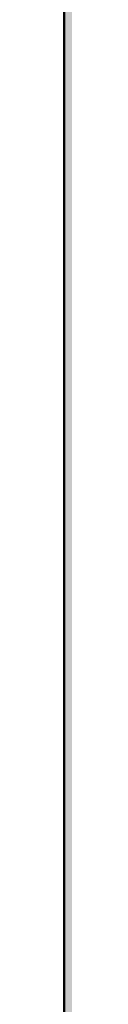
# Model space of a CAD drawing. Units: millimetres. Extents: x 0 to 2267, y 0 to 1823.
# Tile 33 of 256: x 1593.4289 to 1593.4289, y 1226.3857 to 1226.718. Entities that reach past the tile are written whole.
import ezdxf

# ---------------------------------------------------------------- set-up
doc = ezdxf.new("R2010")
doc.units = ezdxf.units.MM
doc.header["$MEASUREMENT"] = 0
doc.layers.add('M-HATC', color=252, linetype='Continuous', lineweight=18)
doc.layers.add('M-OUTL', color=7, linetype='Continuous', lineweight=50)

msp = doc.modelspace()

# ---------------------------------------------------------------- hatches: boundary and pattern name
at = {"layer": 'M-HATC'}
h = msp.add_hatch(color=256, dxfattribs=at)
h.dxf.hatch_style = 1
h.paths.add_polyline_path([(2055.77105, 1603.06204), (1381.08677, 1603.06204), (1381.08677, 1598.06204), (2055.77105, 1598.06204)])
h.paths.add_polyline_path([(2055.77105, 1598.06204), (1381.08677, 1598.06204), (1381.08677, 1593.06204), (2055.77105, 1593.06204)])
h.paths.add_polyline_path([(2051.30737, 1536.76088), (1385.55044, 1536.76088), (1385.55044, 1526.76088), (1387.55044, 1526.76088), (1388.53662, 1525.05276), (1385.33187, 1521.23348), (1385.33187, 1521.22256), (2050.25417, 1522.74913), (2048.32119, 1525.05276), (2049.30737, 1526.76088), (2051.30737, 1526.76088)])
edge = h.paths.add_edge_path()
edge.add_arc((1847.53451, 1379.14917), 135, 222.6030607, 222.8908505, ccw=False)
edge.add_line((1748.16629, 1287.76561), (1683.09212, 1287.76561))
edge.add_arc((1583.7239, 1379.14917), 135, 317.1091495, 317.3969393, ccw=False)
edge.add_arc((1678.9686, 1290.67067), 5, 222.89085, 317.10915, ccw=False)
edge.add_arc((1774.21331, 1379.14917), 135, 222.6030607, 222.8908505, ccw=False)
edge.add_line((1674.84509, 1287.76561), (1609.77092, 1287.76561))
edge.add_arc((1510.4027, 1379.14917), 135, 317.1091495, 317.3969393, ccw=False)
edge.add_arc((1605.6474, 1290.67067), 5, 222.89085, 317.10915, ccw=False)
edge.add_arc((1700.89211, 1379.14917), 135, 222.6030607, 222.8908505, ccw=False)
edge.add_line((1601.52388, 1287.76561), (1536.44972, 1287.76561))
edge.add_arc((1437.08149, 1379.14917), 135, 317.1091495, 317.3969393, ccw=False)
edge.add_arc((1532.3262, 1290.67067), 5, 222.89085, 317.10915, ccw=False)
edge.add_arc((1627.57091, 1379.14917), 135, 222.6030607, 222.8908505, ccw=False)
edge.add_line((1528.20268, 1287.76561), (1505.92891, 1287.76561))
edge.add_spline(control_points=[(1505.92891, 1287.76561), (1504.26224, 1287.76561), (1504.26224, 1282.76561), (1505.92891, 1282.76561)], knot_values=[0, 0, 0, 0, 5, 5, 5, 5], degree=3, periodic=0)
edge.add_line((1505.92891, 1282.76561), (1930.92891, 1282.76561))
edge.add_spline(control_points=[(1930.92891, 1282.76561), (1932.59557, 1282.76561), (1932.59557, 1287.76561), (1930.92891, 1287.76561)], knot_values=[0, 0, 0, 0, 5, 5, 5, 5], degree=3, periodic=0)
edge.add_line((1930.92891, 1287.76561), (1903.05573, 1287.76561))
edge.add_arc((1803.6875, 1379.14917), 135, 317.1091495, 317.3969393, ccw=False)
edge.add_arc((1898.93221, 1290.67067), 5, 222.89085, 317.10915, ccw=False)
edge.add_arc((1994.17691, 1379.14917), 135, 222.6030607, 222.8908505, ccw=False)
edge.add_line((1894.80869, 1287.76561), (1829.73452, 1287.76561))
edge.add_arc((1730.3663, 1379.14917), 135, 317.1091495, 317.3969393, ccw=False)
edge.add_arc((1825.61101, 1290.67067), 5, 222.89085, 317.10915, ccw=False)
edge.add_arc((1920.85571, 1379.14917), 135, 222.6030607, 222.8908505, ccw=False)
edge.add_line((1821.48749, 1287.76561), (1756.41332, 1287.76561))
edge.add_arc((1657.0451, 1379.14917), 135, 317.1091495, 317.3969393, ccw=False)
edge.add_arc((1752.28981, 1290.67067), 5, 222.89085, 317.10915, ccw=False)
edge = h.paths.add_edge_path()
edge.add_spline(control_points=[(1843.42891, 1227.24746), (1845.09557, 1227.24746), (1845.09557, 1232.24746), (1843.42891, 1232.24746)], knot_values=[0, 0, 0, 0, 5, 5, 5, 5], degree=3, periodic=0)
edge.add_line((1843.42891, 1232.24746), (1593.42891, 1232.24746))
edge.add_spline(control_points=[(1593.42891, 1232.24746), (1591.76224, 1232.24746), (1591.76224, 1227.24746), (1593.42891, 1227.24746)], knot_values=[0, 0, 0, 0, 5, 5, 5, 5], degree=3, periodic=0)
edge.add_line((1593.42891, 1227.24746), (1843.42891, 1227.24746))
h.paths.add_polyline_path([(1905.92891, 1127.41706), (1530.92891, 1127.41706, 0.414214), (1520.92891, 1117.41706), (1530.92891, 1117.41706), (1915.92891, 1117.41706, 0.414214)])
edge = h.paths.add_edge_path()
edge.add_arc((1397.08577, 1498.40775), 12.72993, 90.782146, 190.878706, ccw=False)
edge.add_line((1396.912, 1511.13649), (1428.00968, 1511.34875))
edge.add_line((1428.00968, 1511.34875), (1433.00968, 1511.34875))
edge.add_line((1433.00968, 1511.34875), (1434.439, 1511.34875))
edge.add_arc((1419.474, 1498.08041), 20, 41.560995, 74.082109)
edge.add_line((1424.95919, 1517.31353), (1399.93509, 1517.25608))
edge.add_spline(control_points=[(1399.93074, 1517.25607), (1399.88398, 1517.21312), (1399.8328, 1517.16893), (1399.77741, 1517.1236)], knot_values=[11.567499, 11.567499, 11.567499, 11.567499, 11.814249, 11.814249, 11.814249, 11.814249], degree=3, periodic=0)
edge.add_spline(control_points=[(1399.63279, 1517.00986), (1399.58305, 1516.97214), (1399.53072, 1516.93375), (1399.47591, 1516.89474)], knot_values=[11.167718, 11.167718, 11.167718, 11.167718, 11.365188, 11.365188, 11.365188, 11.365188], degree=3, periodic=0)
edge.add_spline(control_points=[(1399.33981, 1516.80007), (1399.15144, 1516.67185), (1398.93836, 1516.5377), (1398.70404, 1516.39942)], knot_values=[10.376405, 10.376405, 10.376405, 10.376405, 11.00994, 11.00994, 11.00994, 11.00994], degree=3, periodic=0)
edge.add_spline(control_points=[(1398.65716, 1516.37187), (1398.57885, 1516.32602), (1398.49825, 1516.27974), (1398.41549, 1516.23309)], knot_values=[10.125175, 10.125175, 10.125175, 10.125175, 10.334406, 10.334406, 10.334406, 10.334406], degree=3, periodic=0)
edge.add_spline(control_points=[(1398.26422, 1516.14874), (1398.19595, 1516.11107), (1398.12634, 1516.07319), (1398.05546, 1516.03513)], knot_values=[9.832246, 9.832246, 9.832246, 9.832246, 9.999658, 9.999658, 9.999658, 9.999658], degree=3, periodic=0)
edge.add_spline(control_points=[(1397.9987, 1516.00476), (1397.73115, 1515.86211), (1397.44602, 1515.71707), (1397.14664, 1515.57138)], knot_values=[9.161808, 9.161808, 9.161808, 9.161808, 9.787769, 9.787769, 9.787769, 9.787769], degree=3, periodic=0)
edge.add_spline(control_points=[(1397.14664, 1515.57138), (1396.84182, 1515.42305), (1396.52223, 1515.27404), (1396.1914, 1515.12621)], knot_values=[8.524455, 8.524455, 8.524455, 8.524455, 9.161808, 9.161808, 9.161808, 9.161808], degree=3, periodic=0)
edge.add_spline(control_points=[(1396.07771, 1515.07565), (1395.98538, 1515.03478), (1395.89222, 1514.99402), (1395.7983, 1514.9534)], knot_values=[8.275193, 8.275193, 8.275193, 8.275193, 8.451726, 8.451726, 8.451726, 8.451726], degree=3, periodic=0)
edge.add_spline(control_points=[(1395.60184, 1514.86912), (1395.49975, 1514.82568), (1395.39685, 1514.78244), (1395.29322, 1514.73944)], knot_values=[7.962917, 7.962917, 7.962917, 7.962917, 8.152764, 8.152764, 8.152764, 8.152764], degree=3, periodic=0)
edge.add_spline(control_points=[(1395.21158, 1514.70568), (1394.82779, 1514.5475), (1394.43452, 1514.39287), (1394.03645, 1514.24422)], knot_values=[7.21254, 7.21254, 7.21254, 7.21254, 7.913148, 7.913148, 7.913148, 7.913148], degree=3, periodic=0)
edge.add_spline(control_points=[(1394.03645, 1514.24422), (1393.70758, 1514.12142), (1393.37544, 1514.0027), (1393.04267, 1513.88945)], knot_values=[6.633733, 6.633733, 6.633733, 6.633733, 7.21254, 7.21254, 7.21254, 7.21254], degree=3, periodic=0)
edge.add_spline(control_points=[(1392.82142, 1513.81499), (1392.71978, 1513.78118), (1392.61815, 1513.74791), (1392.51658, 1513.71521)], knot_values=[6.328796, 6.328796, 6.328796, 6.328796, 6.505493, 6.505493, 6.505493, 6.505493], degree=3, periodic=0)
edge.add_spline(control_points=[(1392.51658, 1513.71521), (1392.31873, 1513.65151), (1392.12116, 1513.59001), (1391.92441, 1513.53098)], knot_values=[5.984605, 5.984605, 5.984605, 5.984605, 6.328796, 6.328796, 6.328796, 6.328796], degree=3, periodic=0)
edge.add_spline(control_points=[(1391.79155, 1513.49146), (1391.31215, 1513.35011), (1390.83842, 1513.22392), (1390.37844, 1513.11711)], knot_values=[5.066697, 5.066697, 5.066697, 5.066697, 5.907055, 5.907055, 5.907055, 5.907055], degree=3, periodic=0)
edge.add_spline(control_points=[(1390.37844, 1513.11711), (1390.17973, 1513.07097), (1389.98359, 1513.02845), (1389.79067, 1512.98988)], knot_values=[4.70367, 4.70367, 4.70367, 4.70367, 5.066695, 5.066695, 5.066695, 5.066695], degree=3, periodic=0)
edge.add_spline(control_points=[(1389.42203, 1512.92036), (1389.24588, 1512.88922), (1389.0729, 1512.86172), (1388.90364, 1512.83814)], knot_values=[4.130571, 4.130571, 4.130571, 4.130571, 4.469816, 4.469816, 4.469816, 4.469816], degree=3, periodic=0)
edge.add_spline(control_points=[(1388.90364, 1512.83814), (1388.59103, 1512.7946), (1388.29108, 1512.76444), (1388.00714, 1512.74941)], knot_values=[3.504031, 3.504031, 3.504031, 3.504031, 4.130571, 4.130571, 4.130571, 4.130571], degree=3, periodic=0)
edge.add_spline(control_points=[(1387.9356, 1512.74593), (1387.85378, 1512.74231), (1387.77334, 1512.73997), (1387.69435, 1512.73898)], knot_values=[3.268866, 3.268866, 3.268866, 3.268866, 3.451164, 3.451164, 3.451164, 3.451164], degree=3, periodic=0)
edge.add_spline(control_points=[(1387.33512, 1512.74426), (1387.20757, 1512.74991), (1387.08472, 1512.7597), (1386.96699, 1512.77385)], knot_values=[2.670686, 2.670686, 2.670686, 2.670686, 2.984, 2.984, 2.984, 2.984], degree=3, periodic=0)
edge.add_spline(control_points=[(1386.83274, 1512.79225), (1386.82093, 1512.79407), (1386.80917, 1512.79594), (1386.79747, 1512.79787)], knot_values=[2.516981, 2.516981, 2.516981, 2.516981, 2.549528, 2.549528, 2.549528, 2.549528], degree=3, periodic=0)
edge.add_spline(control_points=[(1386.45257, 1512.87348), (1386.42573, 1512.88105), (1386.39931, 1512.88895), (1386.3733, 1512.89719)], knot_values=[2.095869, 2.095869, 2.095869, 2.095869, 2.17941, 2.17941, 2.17941, 2.17941], degree=3, periodic=0)
edge.add_spline(control_points=[(1386.06911, 1513.01889), (1386.06338, 1513.02174), (1386.05768, 1513.02463), (1386.05201, 1513.02753)], knot_values=[1.72453, 1.72453, 1.72453, 1.72453, 1.745933, 1.745933, 1.745933, 1.745933], degree=3, periodic=0)
edge.add_arc((1399.474, 1498.08041), 20, 131.824322, 180)
edge.add_arc((1630.33362, 1505.54843), 250.97076, 181.7051759, 236.427975)
edge.add_arc((1605.33992, 1483.30441), 218.7822, 238.660829, 243.3496099)
edge.add_arc((1647.09105, 1510.35917), 262.89859, 183.1298361, 237.8534422, ccw=False)
h.paths.add_polyline_path([(1406.53685, 1391.96444, 0.149382), (1491.55061, 1296.44177, -0.129517)], flags=17)
edge = h.paths.add_edge_path()
edge.add_arc((2037.38381, 1498.08041), 20, 0, 48.265868)
edge.add_spline(control_points=[(2050.69731, 1513.00525), (2050.65121, 1512.98471), (2050.60338, 1512.96554), (2050.55388, 1512.94771)], knot_values=[1.835652, 1.835652, 1.835652, 1.835652, 2.000781, 2.000781, 2.000781, 2.000781], degree=3, periodic=0)
edge.add_spline(control_points=[(2050.46156, 1512.91661), (2050.479, 1512.9221), (2050.49625, 1512.92774), (2050.51332, 1512.93353)], knot_values=[2.045477, 2.045477, 2.045477, 2.045477, 2.101389, 2.101389, 2.101389, 2.101389], degree=3, periodic=0)
edge.add_spline(control_points=[(2050.12896, 1512.83416), (2050.19843, 1512.84734), (2050.26573, 1512.86233), (2050.33075, 1512.87919)], knot_values=[2.237629, 2.237629, 2.237629, 2.237629, 2.435841, 2.435841, 2.435841, 2.435841], degree=3, periodic=0)
edge.add_spline(control_points=[(2050.09463, 1512.82783), (2050.10613, 1512.82989), (2050.11757, 1512.832), (2050.12896, 1512.83416)], knot_values=[2.435841, 2.435841, 2.435841, 2.435841, 2.468321, 2.468321, 2.468321, 2.468321], degree=3, periodic=0)
edge.add_spline(control_points=[(2049.78433, 1512.78511), (2049.85521, 1512.79219), (2049.92435, 1512.80077), (2049.99166, 1512.81088)], knot_values=[2.563852, 2.563852, 2.563852, 2.563852, 2.748541, 2.748541, 2.748541, 2.748541], degree=3, periodic=0)
edge.add_spline(control_points=[(2049.4052, 1512.76169), (2049.5364, 1512.76526), (2049.66292, 1512.77299), (2049.78433, 1512.78511)], knot_values=[2.748541, 2.748541, 2.748541, 2.748541, 3.064882, 3.064882, 3.064882, 3.064882], degree=3, periodic=0)
edge.add_spline(control_points=[(2049.16976, 1512.75968), (2049.23364, 1512.7591), (2049.29654, 1512.7594), (2049.35844, 1512.7606)], knot_values=[3.102309, 3.102309, 3.102309, 3.102309, 3.2503, 3.2503, 3.2503, 3.2503], degree=3, periodic=0)
edge.add_spline(control_points=[(2048.85727, 1512.76911), (2048.96378, 1512.76378), (2049.068, 1512.76061), (2049.16976, 1512.75968)], knot_values=[3.2503, 3.2503, 3.2503, 3.2503, 3.486069, 3.486069, 3.486069, 3.486069], degree=3, periodic=0)
edge.add_spline(control_points=[(2048.69241, 1512.77892), (2048.3729, 1512.80093), (2048.0345, 1512.84106), (2047.68175, 1512.89697)], knot_values=[3.606429, 3.606429, 3.606429, 3.606429, 4.2989, 4.2989, 4.2989, 4.2989], degree=3, periodic=0)
edge.add_spline(control_points=[(2047.68175, 1512.89697), (2047.5458, 1512.91852), (2047.40772, 1512.94241), (2047.26776, 1512.96851)], knot_values=[4.2989, 4.2989, 4.2989, 4.2989, 4.565769, 4.565769, 4.565769, 4.565769], degree=3, periodic=0)
edge.add_spline(control_points=[(2047.26776, 1512.96851), (2047.14494, 1512.99141), (2047.02067, 1513.01601), (2046.89514, 1513.04223)], knot_values=[4.565769, 4.565769, 4.565769, 4.565769, 4.799971, 4.799971, 4.799971, 4.799971], degree=3, periodic=0)
edge.add_spline(control_points=[(2046.89514, 1513.04223), (2046.52865, 1513.11875), (2046.15135, 1513.20899), (2045.7676, 1513.31068)], knot_values=[4.799971, 4.799971, 4.799971, 4.799971, 5.483718, 5.483718, 5.483718, 5.483718], degree=3, periodic=0)
edge.add_spline(control_points=[(2045.7676, 1513.31068), (2045.3724, 1513.41539), (2044.97036, 1513.53225), (2044.56625, 1513.65876)], knot_values=[5.483718, 5.483718, 5.483718, 5.483718, 6.187866, 6.187866, 6.187866, 6.187866], degree=3, periodic=0)
edge.add_spline(control_points=[(2044.56625, 1513.65876), (2044.41491, 1513.70614), (2044.26329, 1513.75487), (2044.11163, 1513.80482)], knot_values=[6.187866, 6.187866, 6.187866, 6.187866, 6.451551, 6.451551, 6.451551, 6.451551], degree=3, periodic=0)
edge.add_spline(control_points=[(2044.11163, 1513.80482), (2043.99666, 1513.84269), (2043.88167, 1513.88126), (2043.76676, 1513.92048)], knot_values=[6.451551, 6.451551, 6.451551, 6.451551, 6.651434, 6.651434, 6.651434, 6.651434], degree=3, periodic=0)
edge.add_spline(control_points=[(2043.76676, 1513.92048), (2043.37157, 1514.05536), (2042.97738, 1514.19789), (2042.58863, 1514.34575)], knot_values=[6.651434, 6.651434, 6.651434, 6.651434, 7.338879, 7.338879, 7.338879, 7.338879], degree=3, periodic=0)
edge.add_spline(control_points=[(2042.58863, 1514.34575), (2042.16431, 1514.50715), (2041.74647, 1514.67491), (2041.34086, 1514.84603)], knot_values=[7.338879, 7.338879, 7.338879, 7.338879, 8.089209, 8.089209, 8.089209, 8.089209], degree=3, periodic=0)
edge.add_spline(control_points=[(2041.34086, 1514.84603), (2041.1028, 1514.94647), (2040.86896, 1515.04806), (2040.64049, 1515.1502)], knot_values=[8.089209, 8.089209, 8.089209, 8.089209, 8.529587, 8.529587, 8.529587, 8.529587], degree=3, periodic=0)
edge.add_spline(control_points=[(2040.50999, 1515.20887), (2040.08238, 1515.40218), (2039.67475, 1515.59705), (2039.29495, 1515.78939)], knot_values=[8.613818, 8.613818, 8.613818, 8.613818, 9.44571, 9.44571, 9.44571, 9.44571], degree=3, periodic=0)
edge.add_spline(control_points=[(2039.29495, 1515.78939), (2039.0618, 1515.90746), (2038.83914, 1516.02458), (2038.62878, 1516.1398)], knot_values=[9.44571, 9.44571, 9.44571, 9.44571, 9.956404, 9.956404, 9.956404, 9.956404], degree=3, periodic=0)
edge.add_spline(control_points=[(2038.62878, 1516.1398), (2038.51874, 1516.20007), (2038.41207, 1516.25982), (2038.30903, 1516.31891)], knot_values=[9.956404, 9.956404, 9.956404, 9.956404, 10.223542, 10.223542, 10.223542, 10.223542], degree=3, periodic=0)
edge.add_spline(control_points=[(2038.30903, 1516.31891), (2038.21377, 1516.37354), (2038.12161, 1516.42762), (2038.03275, 1516.48102)], knot_values=[10.223542, 10.223542, 10.223542, 10.223542, 10.47051, 10.47051, 10.47051, 10.47051], degree=3, periodic=0)
edge.add_spline(control_points=[(2038.03275, 1516.48102), (2037.78552, 1516.62961), (2037.56388, 1516.77304), (2037.37225, 1516.909)], knot_values=[10.47051, 10.47051, 10.47051, 10.47051, 11.15767, 11.15767, 11.15767, 11.15767], degree=3, periodic=0)
edge.add_spline(control_points=[(2037.37225, 1516.909), (2037.27893, 1516.9752), (2037.19274, 1517.03963), (2037.11417, 1517.10203)], knot_values=[11.15767, 11.15767, 11.15767, 11.15767, 11.49227, 11.49227, 11.49227, 11.49227], degree=3, periodic=0)
edge.add_spline(control_points=[(2036.85638, 1517.32585), (2036.91481, 1517.26923), (2036.98143, 1517.21027), (2037.05573, 1517.14922)], knot_values=[11.577341, 11.577341, 11.577341, 11.577341, 11.91035, 11.91035, 11.91035, 11.91035], degree=3, periodic=0)
edge.add_spline(control_points=[(2036.80739, 1517.37475), (2036.82301, 1517.35865), (2036.83935, 1517.34235), (2036.85638, 1517.32585)], knot_values=[11.91035, 11.91035, 11.91035, 11.91035, 12.007402, 12.007402, 12.007402, 12.007402], degree=3, periodic=0)
edge.add_spline(control_points=[(2036.70167, 1517.494), (2036.71042, 1517.48299), (2036.71958, 1517.47185), (2036.72913, 1517.4606)], knot_values=[12.184155, 12.184155, 12.184155, 12.184155, 12.255409, 12.255409, 12.255409, 12.255409], degree=3, periodic=0)
edge.add_spline(control_points=[(2036.6159, 1517.6205), (2036.61998, 1517.61304), (2036.6243, 1517.6055), (2036.62885, 1517.59789)], knot_values=[12.487913, 12.487913, 12.487913, 12.487913, 12.541035, 12.541035, 12.541035, 12.541035], degree=3, periodic=0)
edge.add_spline(control_points=[(2036.56349, 1517.78599), (2036.56372, 1517.77936), (2036.56423, 1517.77264), (2036.56502, 1517.76582)], knot_values=[12.911761, 12.911761, 12.911761, 12.911761, 12.968286, 12.968286, 12.968286, 12.968286], degree=3, periodic=0)
edge.add_spline(control_points=[(2036.61663, 1517.93042), (2036.61248, 1517.92586), (2036.60857, 1517.92121), (2036.60491, 1517.91648)], knot_values=[13.382527, 13.382527, 13.382527, 13.382527, 13.433791, 13.433791, 13.433791, 13.433791], degree=3, periodic=0)
edge.add_spline(control_points=[(2036.74902, 1518.01695), (2036.73613, 1518.0116), (2036.72393, 1518.00601), (2036.71242, 1518.00018)], knot_values=[13.726299, 13.726299, 13.726299, 13.726299, 13.809928, 13.809928, 13.809928, 13.809928], degree=3, periodic=0)
edge.add_spline(control_points=[(2036.86043, 1518.05285), (2036.83863, 1518.04743), (2036.81809, 1518.04156), (2036.79879, 1518.03526)], knot_values=[13.910887, 13.910887, 13.910887, 13.910887, 14.02153, 14.02153, 14.02153, 14.02153], degree=3, periodic=0)
edge.add_line((2036.96387, 1518.08041), (2032.38381, 1518.08041))
edge.add_line((2032.38381, 1518.08041), (2027.38381, 1518.08041))
edge.add_line((2027.38381, 1518.08041), (2022.38381, 1518.08041))
edge.add_line((2022.38381, 1518.08041), (2017.38381, 1518.08041))
edge.add_arc((2017.38381, 1498.08041), 20, 90, 138.439005)
edge.add_line((2002.41881, 1511.34875), (2003.84813, 1511.34875))
edge.add_line((2003.84813, 1511.34875), (2008.84813, 1511.34875))
edge.add_line((2008.84813, 1511.34875), (2039.77204, 1511.13768))
edge.add_arc((2039.77204, 1498.40775), 12.72993, -10.878706, 90, ccw=False)
edge.add_arc((1789.76676, 1510.35917), 262.89859, 302.1465578, 356.8701639, ccw=False)
edge.add_arc((1831.51789, 1483.30441), 218.7822, 296.6503901, 301.339171)
edge.add_arc((1806.52419, 1505.54843), 250.97076, 303.572025, 358.2948241)
h.paths.add_polyline_path([(2030.32096, 1391.96444, -0.129517), (1945.3072, 1296.44177, 0.149382)], flags=17)
edge = h.paths.add_edge_path()
edge.add_spline(control_points=[(2037.2464, 1518.08209), (2037.28977, 1518.08098), (2037.33555, 1518.08041), (2037.3838, 1518.08041)], knot_values=[0.000012, 0.000012, 0.000012, 0.000012, 0.144754, 0.144754, 0.144754, 0.144754], degree=3, periodic=0)
edge.add_line((2037.33571, 1518.08041), (2037.00963, 1518.08041))
edge.add_spline(control_points=[(2037.00963, 1518.08041), (2036.98217, 1518.07678), (2036.95605, 1518.07266), (2036.93124, 1518.06808)], knot_values=[14.13465, 14.13465, 14.13465, 14.13465, 14.247197, 14.247197, 14.247197, 14.247197], degree=3, periodic=0)
edge.add_spline(control_points=[(2036.93124, 1518.06808), (2036.92764, 1518.06741), (2036.92407, 1518.06674), (2036.92053, 1518.06605)], knot_values=[14.118315, 14.118315, 14.118315, 14.118315, 14.13465, 14.13465, 14.13465, 14.13465], degree=3, periodic=0)
edge.add_spline(control_points=[(2036.92053, 1518.06605), (2036.9118, 1518.06436), (2036.90323, 1518.06262), (2036.89484, 1518.06081)], knot_values=[14.078086, 14.078086, 14.078086, 14.078086, 14.118315, 14.118315, 14.118315, 14.118315], degree=3, periodic=0)
edge.add_spline(control_points=[(2036.89484, 1518.06081), (2036.88304, 1518.05827), (2036.87157, 1518.05562), (2036.86043, 1518.05285)], knot_values=[14.02153, 14.02153, 14.02153, 14.02153, 14.078086, 14.078086, 14.078086, 14.078086], degree=3, periodic=0)
edge.add_spline(control_points=[(2036.86043, 1518.05285), (2036.83863, 1518.04743), (2036.81809, 1518.04156), (2036.79879, 1518.03526)], knot_values=[13.910887, 13.910887, 13.910887, 13.910887, 14.02153, 14.02153, 14.02153, 14.02153], degree=3, periodic=0)
edge.add_spline(control_points=[(2036.79879, 1518.03526), (2036.79809, 1518.03504), (2036.7974, 1518.03481), (2036.79671, 1518.03458)], knot_values=[13.906906, 13.906906, 13.906906, 13.906906, 13.910887, 13.910887, 13.910887, 13.910887], degree=3, periodic=0)
edge.add_spline(control_points=[(2036.79671, 1518.03458), (2036.78819, 1518.03178), (2036.77991, 1518.02888), (2036.77187, 1518.02591)], knot_values=[13.857826, 13.857826, 13.857826, 13.857826, 13.906906, 13.906906, 13.906906, 13.906906], degree=3, periodic=0)
edge.add_spline(control_points=[(2036.77187, 1518.02591), (2036.76402, 1518.023), (2036.75641, 1518.02002), (2036.74902, 1518.01695)], knot_values=[13.809928, 13.809928, 13.809928, 13.809928, 13.857826, 13.857826, 13.857826, 13.857826], degree=3, periodic=0)
edge.add_spline(control_points=[(2036.74902, 1518.01695), (2036.73613, 1518.0116), (2036.72393, 1518.00601), (2036.71242, 1518.00018)], knot_values=[13.726299, 13.726299, 13.726299, 13.726299, 13.809928, 13.809928, 13.809928, 13.809928], degree=3, periodic=0)
edge.add_spline(control_points=[(2036.71242, 1518.00018), (2036.71211, 1518.00002), (2036.71179, 1517.99986), (2036.71147, 1517.99969)], knot_values=[13.723993, 13.723993, 13.723993, 13.723993, 13.726299, 13.726299, 13.726299, 13.726299], degree=3, periodic=0)
edge.add_spline(control_points=[(2036.71147, 1517.99969), (2036.70634, 1517.99708), (2036.70134, 1517.99441), (2036.69648, 1517.9917)], knot_values=[13.686536, 13.686536, 13.686536, 13.686536, 13.723993, 13.723993, 13.723993, 13.723993], degree=3, periodic=0)
edge.add_spline(control_points=[(2036.69648, 1517.9917), (2036.6919, 1517.98914), (2036.68744, 1517.98654), (2036.6831, 1517.9839)], knot_values=[13.651251, 13.651251, 13.651251, 13.651251, 13.686536, 13.686536, 13.686536, 13.686536], degree=3, periodic=0)
edge.add_spline(control_points=[(2036.6831, 1517.9839), (2036.67641, 1517.97983), (2036.67001, 1517.97566), (2036.6639, 1517.97139)], knot_values=[13.596804, 13.596804, 13.596804, 13.596804, 13.651251, 13.651251, 13.651251, 13.651251], degree=3, periodic=0)
edge.add_spline(control_points=[(2036.6639, 1517.97139), (2036.66358, 1517.97117), (2036.66326, 1517.97094), (2036.66294, 1517.97072)], knot_values=[13.593956, 13.593956, 13.593956, 13.593956, 13.596804, 13.596804, 13.596804, 13.596804], degree=3, periodic=0)
edge.add_spline(control_points=[(2036.66294, 1517.97072), (2036.6603, 1517.96886), (2036.65771, 1517.96698), (2036.65518, 1517.96509)], knot_values=[13.570322, 13.570322, 13.570322, 13.570322, 13.593956, 13.593956, 13.593956, 13.593956], degree=3, periodic=0)
edge.add_spline(control_points=[(2036.65518, 1517.96509), (2036.65251, 1517.9631), (2036.64991, 1517.96108), (2036.64737, 1517.95905)], knot_values=[13.545477, 13.545477, 13.545477, 13.545477, 13.570322, 13.570322, 13.570322, 13.570322], degree=3, periodic=0)
edge.add_spline(control_points=[(2036.64737, 1517.95905), (2036.64721, 1517.95892), (2036.64705, 1517.9588), (2036.64689, 1517.95867)], knot_values=[13.543931, 13.543931, 13.543931, 13.543931, 13.545477, 13.545477, 13.545477, 13.545477], degree=3, periodic=0)
edge.add_spline(control_points=[(2036.64689, 1517.95867), (2036.64121, 1517.95411), (2036.63582, 1517.94945), (2036.63073, 1517.94468)], knot_values=[13.488237, 13.488237, 13.488237, 13.488237, 13.543931, 13.543931, 13.543931, 13.543931], degree=3, periodic=0)
edge.add_spline(control_points=[(2036.63073, 1517.94468), (2036.62817, 1517.94229), (2036.62569, 1517.93988), (2036.62329, 1517.93744)], knot_values=[13.460307, 13.460307, 13.460307, 13.460307, 13.488237, 13.488237, 13.488237, 13.488237], degree=3, periodic=0)
edge.add_spline(control_points=[(2036.62329, 1517.93744), (2036.62151, 1517.93564), (2036.61978, 1517.93383), (2036.61809, 1517.932)], knot_values=[13.439712, 13.439712, 13.439712, 13.439712, 13.460307, 13.460307, 13.460307, 13.460307], degree=3, periodic=0)
edge.add_spline(control_points=[(2036.61809, 1517.932), (2036.6176, 1517.93147), (2036.61711, 1517.93095), (2036.61663, 1517.93042)], knot_values=[13.433791, 13.433791, 13.433791, 13.433791, 13.439712, 13.439712, 13.439712, 13.439712], degree=3, periodic=0)
edge.add_spline(control_points=[(2036.61663, 1517.93042), (2036.61248, 1517.92586), (2036.60857, 1517.92121), (2036.60491, 1517.91648)], knot_values=[13.382527, 13.382527, 13.382527, 13.382527, 13.433791, 13.433791, 13.433791, 13.433791], degree=3, periodic=0)
edge.add_spline(control_points=[(2036.60491, 1517.91648), (2036.60258, 1517.91347), (2036.60036, 1517.91044), (2036.59824, 1517.90737)], knot_values=[13.350017, 13.350017, 13.350017, 13.350017, 13.382527, 13.382527, 13.382527, 13.382527], degree=3, periodic=0)
edge.add_spline(control_points=[(2036.59824, 1517.90737), (2036.59718, 1517.90585), (2036.59616, 1517.90433), (2036.59515, 1517.90279)], knot_values=[13.333922, 13.333922, 13.333922, 13.333922, 13.350017, 13.350017, 13.350017, 13.350017], degree=3, periodic=0)
edge.add_spline(control_points=[(2036.59515, 1517.90279), (2036.59452, 1517.90183), (2036.5939, 1517.90086), (2036.59329, 1517.89989)], knot_values=[13.323828, 13.323828, 13.323828, 13.323828, 13.333922, 13.333922, 13.333922, 13.333922], degree=3, periodic=0)
edge.add_spline(control_points=[(2036.59329, 1517.89989), (2036.59049, 1517.89545), (2036.5879, 1517.89094), (2036.5855, 1517.88637)], knot_values=[13.277545, 13.277545, 13.277545, 13.277545, 13.323828, 13.323828, 13.323828, 13.323828], degree=3, periodic=0)
edge.add_spline(control_points=[(2036.5855, 1517.88637), (2036.58355, 1517.88267), (2036.58174, 1517.87892), (2036.58006, 1517.87513)], knot_values=[13.240119, 13.240119, 13.240119, 13.240119, 13.277545, 13.277545, 13.277545, 13.277545], degree=3, periodic=0)
edge.add_spline(control_points=[(2036.58006, 1517.87513), (2036.57952, 1517.87393), (2036.579, 1517.87272), (2036.57849, 1517.87151)], knot_values=[13.228211, 13.228211, 13.228211, 13.228211, 13.240119, 13.240119, 13.240119, 13.240119], degree=3, periodic=0)
edge.add_spline(control_points=[(2036.57849, 1517.87151), (2036.57796, 1517.87023), (2036.57744, 1517.86896), (2036.57693, 1517.86767)], knot_values=[13.215717, 13.215717, 13.215717, 13.215717, 13.228211, 13.228211, 13.228211, 13.228211], degree=3, periodic=0)
edge.add_spline(control_points=[(2036.57693, 1517.86767), (2036.57548, 1517.86399), (2036.57414, 1517.86027), (2036.57293, 1517.85651)], knot_values=[13.179847, 13.179847, 13.179847, 13.179847, 13.215717, 13.215717, 13.215717, 13.215717], degree=3, periodic=0)
edge.add_spline(control_points=[(2036.57293, 1517.85651), (2036.5713, 1517.8515), (2036.56989, 1517.84641), (2036.56868, 1517.84126)], knot_values=[13.132017, 13.132017, 13.132017, 13.132017, 13.179847, 13.179847, 13.179847, 13.179847], degree=3, periodic=0)
edge.add_spline(control_points=[(2036.56868, 1517.84126), (2036.56844, 1517.84023), (2036.56821, 1517.8392), (2036.56798, 1517.83817)], knot_values=[13.122482, 13.122482, 13.122482, 13.122482, 13.132017, 13.132017, 13.132017, 13.132017], degree=3, periodic=0)
edge.add_spline(control_points=[(2036.56798, 1517.83817), (2036.56758, 1517.83634), (2036.56721, 1517.8345), (2036.56687, 1517.83266)], knot_values=[13.105592, 13.105592, 13.105592, 13.105592, 13.122482, 13.122482, 13.122482, 13.122482], degree=3, periodic=0)
edge.add_spline(control_points=[(2036.56687, 1517.83266), (2036.56622, 1517.82921), (2036.56567, 1517.82574), (2036.5652, 1517.82223)], knot_values=[13.074063, 13.074063, 13.074063, 13.074063, 13.105592, 13.105592, 13.105592, 13.105592], degree=3, periodic=0)
edge.add_spline(control_points=[(2036.5652, 1517.82223), (2036.5652, 1517.82223), (2036.5652, 1517.82223), (2036.5652, 1517.82223)], knot_values=[13.074043, 13.074043, 13.074043, 13.074043, 13.074063, 13.074063, 13.074063, 13.074063], degree=3, periodic=0)
edge.add_spline(control_points=[(2036.5652, 1517.82223), (2036.56443, 1517.81643), (2036.5639, 1517.81055), (2036.56361, 1517.8046)], knot_values=[13.021884, 13.021884, 13.021884, 13.021884, 13.074043, 13.074043, 13.074043, 13.074043], degree=3, periodic=0)
edge.add_spline(control_points=[(2036.56361, 1517.8046), (2036.56358, 1517.80401), (2036.56356, 1517.80342), (2036.56353, 1517.80283)], knot_values=[13.01674, 13.01674, 13.01674, 13.01674, 13.021884, 13.021884, 13.021884, 13.021884], degree=3, periodic=0)
edge.add_spline(control_points=[(2036.56353, 1517.80283), (2036.56344, 1517.80051), (2036.56338, 1517.79817), (2036.56336, 1517.79582)], knot_values=[12.996438, 12.996438, 12.996438, 12.996438, 13.01674, 13.01674, 13.01674, 13.01674], degree=3, periodic=0)
edge.add_spline(control_points=[(2036.56336, 1517.79582), (2036.56334, 1517.79257), (2036.56338, 1517.78929), (2036.56349, 1517.78599)], knot_values=[12.968286, 12.968286, 12.968286, 12.968286, 12.996438, 12.996438, 12.996438, 12.996438], degree=3, periodic=0)
edge.add_spline(control_points=[(2036.56349, 1517.78599), (2036.56372, 1517.77936), (2036.56423, 1517.77264), (2036.56502, 1517.76582)], knot_values=[12.911761, 12.911761, 12.911761, 12.911761, 12.968286, 12.968286, 12.968286, 12.968286], degree=3, periodic=0)
edge.add_spline(control_points=[(2036.56502, 1517.76582), (2036.56503, 1517.76573), (2036.56504, 1517.76564), (2036.56505, 1517.76555)], knot_values=[12.911017, 12.911017, 12.911017, 12.911017, 12.911761, 12.911761, 12.911761, 12.911761], degree=3, periodic=0)
edge.add_spline(control_points=[(2036.56505, 1517.76555), (2036.56541, 1517.76245), (2036.56583, 1517.75933), (2036.56631, 1517.75619)], knot_values=[12.88528, 12.88528, 12.88528, 12.88528, 12.911017, 12.911017, 12.911017, 12.911017], degree=3, periodic=0)
edge.add_spline(control_points=[(2036.56631, 1517.75619), (2036.56673, 1517.75341), (2036.5672, 1517.75062), (2036.56771, 1517.74782)], knot_values=[12.862519, 12.862519, 12.862519, 12.862519, 12.88528, 12.88528, 12.88528, 12.88528], degree=3, periodic=0)
edge.add_spline(control_points=[(2036.56771, 1517.74782), (2036.56779, 1517.74737), (2036.56788, 1517.74692), (2036.56796, 1517.74647)], knot_values=[12.858885, 12.858885, 12.858885, 12.858885, 12.862519, 12.862519, 12.862519, 12.862519], degree=3, periodic=0)
edge.add_spline(control_points=[(2036.56796, 1517.74647), (2036.5692, 1517.73986), (2036.57069, 1517.73316), (2036.57243, 1517.72638)], knot_values=[12.8053, 12.8053, 12.8053, 12.8053, 12.858885, 12.858885, 12.858885, 12.858885], degree=3, periodic=0)
edge.add_spline(control_points=[(2036.57243, 1517.72638), (2036.5734, 1517.72257), (2036.57446, 1517.71874), (2036.57559, 1517.71488)], knot_values=[12.775176, 12.775176, 12.775176, 12.775176, 12.8053, 12.8053, 12.8053, 12.8053], degree=3, periodic=0)
edge.add_spline(control_points=[(2036.57559, 1517.71488), (2036.57628, 1517.71252), (2036.577, 1517.71015), (2036.57775, 1517.70778)], knot_values=[12.756759, 12.756759, 12.756759, 12.756759, 12.775176, 12.775176, 12.775176, 12.775176], degree=3, periodic=0)
edge.add_spline(control_points=[(2036.57775, 1517.70778), (2036.57808, 1517.70674), (2036.57841, 1517.7057), (2036.57875, 1517.70466)], knot_values=[12.748742, 12.748742, 12.748742, 12.748742, 12.756759, 12.756759, 12.756759, 12.756759], degree=3, periodic=0)
edge.add_spline(control_points=[(2036.57875, 1517.70466), (2036.58082, 1517.6983), (2036.58309, 1517.69187), (2036.58557, 1517.68537)], knot_values=[12.69959, 12.69959, 12.69959, 12.69959, 12.748742, 12.748742, 12.748742, 12.748742], degree=3, periodic=0)
edge.add_spline(control_points=[(2036.58557, 1517.68537), (2036.58762, 1517.68001), (2036.5898, 1517.6746), (2036.59213, 1517.66916)], knot_values=[12.659038, 12.659038, 12.659038, 12.659038, 12.69959, 12.69959, 12.69959, 12.69959], degree=3, periodic=0)
edge.add_spline(control_points=[(2036.59213, 1517.66916), (2036.59397, 1517.66482), (2036.59591, 1517.66047), (2036.59793, 1517.65608)], knot_values=[12.626806, 12.626806, 12.626806, 12.626806, 12.659038, 12.659038, 12.659038, 12.659038], degree=3, periodic=0)
edge.add_spline(control_points=[(2036.59793, 1517.65608), (2036.59839, 1517.65507), (2036.59886, 1517.65406), (2036.59934, 1517.65305)], knot_values=[12.619394, 12.619394, 12.619394, 12.619394, 12.626806, 12.626806, 12.626806, 12.626806], degree=3, periodic=0)
edge.add_spline(control_points=[(2036.59934, 1517.65305), (2036.60435, 1517.64236), (2036.60987, 1517.63151), (2036.61589, 1517.6205)], knot_values=[12.541039, 12.541039, 12.541039, 12.541039, 12.619394, 12.619394, 12.619394, 12.619394], degree=3, periodic=0)
edge.add_spline(control_points=[(2036.61589, 1517.6205), (2036.61589, 1517.6205), (2036.6159, 1517.6205), (2036.6159, 1517.6205)], knot_values=[12.541035, 12.541035, 12.541035, 12.541035, 12.541039, 12.541039, 12.541039, 12.541039], degree=3, periodic=0)
edge.add_spline(control_points=[(2036.6159, 1517.6205), (2036.61998, 1517.61304), (2036.6243, 1517.6055), (2036.62885, 1517.59789)], knot_values=[12.487913, 12.487913, 12.487913, 12.487913, 12.541035, 12.541035, 12.541035, 12.541035], degree=3, periodic=0)
edge.add_spline(control_points=[(2036.62885, 1517.59789), (2036.63261, 1517.5916), (2036.63653, 1517.58526), (2036.64061, 1517.57888)], knot_values=[12.443982, 12.443982, 12.443982, 12.443982, 12.487913, 12.487913, 12.487913, 12.487913], degree=3, periodic=0)
edge.add_spline(control_points=[(2036.64061, 1517.57888), (2036.64144, 1517.57757), (2036.64228, 1517.57626), (2036.64313, 1517.57495)], knot_values=[12.434996, 12.434996, 12.434996, 12.434996, 12.443982, 12.443982, 12.443982, 12.443982], degree=3, periodic=0)
edge.add_spline(control_points=[(2036.64313, 1517.57495), (2036.65306, 1517.55958), (2036.66389, 1517.54394), (2036.6756, 1517.52803)], knot_values=[12.329647, 12.329647, 12.329647, 12.329647, 12.434996, 12.434996, 12.434996, 12.434996], degree=3, periodic=0)
edge.add_spline(control_points=[(2036.6756, 1517.52803), (2036.68385, 1517.51682), (2036.69254, 1517.50548), (2036.70167, 1517.494)], knot_values=[12.255409, 12.255409, 12.255409, 12.255409, 12.329647, 12.329647, 12.329647, 12.329647], degree=3, periodic=0)
edge.add_spline(control_points=[(2036.70167, 1517.494), (2036.71042, 1517.48299), (2036.71958, 1517.47185), (2036.72913, 1517.4606)], knot_values=[12.184155, 12.184155, 12.184155, 12.184155, 12.255409, 12.255409, 12.255409, 12.255409], degree=3, periodic=0)
edge.add_spline(control_points=[(2036.72913, 1517.4606), (2036.74363, 1517.44352), (2036.75904, 1517.42617), (2036.77534, 1517.40855)], knot_values=[12.075961, 12.075961, 12.075961, 12.075961, 12.184155, 12.184155, 12.184155, 12.184155], degree=3, periodic=0)
edge.add_spline(control_points=[(2036.77534, 1517.40855), (2036.77631, 1517.4075), (2036.77729, 1517.40645), (2036.77827, 1517.40539)], knot_values=[12.069502, 12.069502, 12.069502, 12.069502, 12.075961, 12.075961, 12.075961, 12.075961], degree=3, periodic=0)
edge.add_spline(control_points=[(2036.77827, 1517.40539), (2036.78768, 1517.39526), (2036.79739, 1517.38505), (2036.80739, 1517.37475)], knot_values=[12.007402, 12.007402, 12.007402, 12.007402, 12.069502, 12.069502, 12.069502, 12.069502], degree=3, periodic=0)
edge.add_spline(control_points=[(2036.80739, 1517.37475), (2036.82301, 1517.35865), (2036.83935, 1517.34235), (2036.85638, 1517.32585)], knot_values=[11.91035, 11.91035, 11.91035, 11.91035, 12.007402, 12.007402, 12.007402, 12.007402], degree=3, periodic=0)
edge.add_spline(control_points=[(2036.85638, 1517.32585), (2036.91481, 1517.26923), (2036.98143, 1517.21027), (2037.05573, 1517.14922)], knot_values=[11.577341, 11.577341, 11.577341, 11.577341, 11.91035, 11.91035, 11.91035, 11.91035], degree=3, periodic=0)
edge.add_spline(control_points=[(2037.05573, 1517.14922), (2037.07471, 1517.13362), (2037.0942, 1517.11789), (2037.11417, 1517.10203)], knot_values=[11.49227, 11.49227, 11.49227, 11.49227, 11.577341, 11.577341, 11.577341, 11.577341], degree=3, periodic=0)
edge.add_spline(control_points=[(2037.11417, 1517.10203), (2037.19274, 1517.03963), (2037.27893, 1516.9752), (2037.37225, 1516.909)], knot_values=[11.15767, 11.15767, 11.15767, 11.15767, 11.49227, 11.49227, 11.49227, 11.49227], degree=3, periodic=0)
edge.add_spline(control_points=[(2037.37225, 1516.909), (2037.56388, 1516.77304), (2037.78552, 1516.62961), (2038.03275, 1516.48102)], knot_values=[10.47051, 10.47051, 10.47051, 10.47051, 11.15767, 11.15767, 11.15767, 11.15767], degree=3, periodic=0)
edge.add_spline(control_points=[(2038.03275, 1516.48102), (2038.12161, 1516.42762), (2038.21377, 1516.37354), (2038.30903, 1516.31891)], knot_values=[10.223542, 10.223542, 10.223542, 10.223542, 10.47051, 10.47051, 10.47051, 10.47051], degree=3, periodic=0)
edge.add_spline(control_points=[(2038.30903, 1516.31891), (2038.41207, 1516.25982), (2038.51874, 1516.20007), (2038.62878, 1516.1398)], knot_values=[9.956404, 9.956404, 9.956404, 9.956404, 10.223542, 10.223542, 10.223542, 10.223542], degree=3, periodic=0)
edge.add_spline(control_points=[(2038.62878, 1516.1398), (2038.83914, 1516.02458), (2039.0618, 1515.90746), (2039.29495, 1515.78939)], knot_values=[9.44571, 9.44571, 9.44571, 9.44571, 9.956404, 9.956404, 9.956404, 9.956404], degree=3, periodic=0)
edge.add_spline(control_points=[(2039.29495, 1515.78939), (2039.67475, 1515.59705), (2040.08238, 1515.40218), (2040.50999, 1515.20887)], knot_values=[8.613818, 8.613818, 8.613818, 8.613818, 9.44571, 9.44571, 9.44571, 9.44571], degree=3, periodic=0)
edge.add_spline(control_points=[(2040.50999, 1515.20887), (2040.55329, 1515.1893), (2040.59679, 1515.16974), (2040.64049, 1515.1502)], knot_values=[8.529587, 8.529587, 8.529587, 8.529587, 8.613818, 8.613818, 8.613818, 8.613818], degree=3, periodic=0)
edge.add_spline(control_points=[(2040.64049, 1515.1502), (2040.86896, 1515.04806), (2041.1028, 1514.94647), (2041.34086, 1514.84603)], knot_values=[8.089209, 8.089209, 8.089209, 8.089209, 8.529587, 8.529587, 8.529587, 8.529587], degree=3, periodic=0)
edge.add_spline(control_points=[(2041.34086, 1514.84603), (2041.74647, 1514.67491), (2042.16431, 1514.50715), (2042.58863, 1514.34575)], knot_values=[7.338879, 7.338879, 7.338879, 7.338879, 8.089209, 8.089209, 8.089209, 8.089209], degree=3, periodic=0)
edge.add_spline(control_points=[(2042.58863, 1514.34575), (2042.97738, 1514.19789), (2043.37157, 1514.05536), (2043.76676, 1513.92048)], knot_values=[6.651434, 6.651434, 6.651434, 6.651434, 7.338879, 7.338879, 7.338879, 7.338879], degree=3, periodic=0)
edge.add_spline(control_points=[(2043.76676, 1513.92048), (2043.88167, 1513.88126), (2043.99666, 1513.84269), (2044.11163, 1513.80482)], knot_values=[6.451551, 6.451551, 6.451551, 6.451551, 6.651434, 6.651434, 6.651434, 6.651434], degree=3, periodic=0)
edge.add_spline(control_points=[(2044.11163, 1513.80482), (2044.26329, 1513.75487), (2044.41491, 1513.70614), (2044.56625, 1513.65876)], knot_values=[6.187866, 6.187866, 6.187866, 6.187866, 6.451551, 6.451551, 6.451551, 6.451551], degree=3, periodic=0)
edge.add_spline(control_points=[(2044.56625, 1513.65876), (2044.97036, 1513.53225), (2045.3724, 1513.41539), (2045.7676, 1513.31068)], knot_values=[5.483718, 5.483718, 5.483718, 5.483718, 6.187866, 6.187866, 6.187866, 6.187866], degree=3, periodic=0)
edge.add_spline(control_points=[(2045.7676, 1513.31068), (2046.15135, 1513.20899), (2046.52865, 1513.11875), (2046.89514, 1513.04223)], knot_values=[4.799971, 4.799971, 4.799971, 4.799971, 5.483718, 5.483718, 5.483718, 5.483718], degree=3, periodic=0)
edge.add_spline(control_points=[(2046.89514, 1513.04223), (2047.02067, 1513.01601), (2047.14494, 1512.99141), (2047.26776, 1512.96851)], knot_values=[4.565769, 4.565769, 4.565769, 4.565769, 4.799971, 4.799971, 4.799971, 4.799971], degree=3, periodic=0)
edge.add_spline(control_points=[(2047.26776, 1512.96851), (2047.40772, 1512.94241), (2047.5458, 1512.91852), (2047.68175, 1512.89697)], knot_values=[4.2989, 4.2989, 4.2989, 4.2989, 4.565769, 4.565769, 4.565769, 4.565769], degree=3, periodic=0)
edge.add_spline(control_points=[(2047.68175, 1512.89697), (2048.0345, 1512.84106), (2048.3729, 1512.80093), (2048.69241, 1512.77892)], knot_values=[3.606429, 3.606429, 3.606429, 3.606429, 4.2989, 4.2989, 4.2989, 4.2989], degree=3, periodic=0)
edge.add_spline(control_points=[(2048.69241, 1512.77892), (2048.74794, 1512.7751), (2048.8029, 1512.77182), (2048.85727, 1512.76911)], knot_values=[3.486069, 3.486069, 3.486069, 3.486069, 3.606429, 3.606429, 3.606429, 3.606429], degree=3, periodic=0)
edge.add_spline(control_points=[(2048.85727, 1512.76911), (2048.96378, 1512.76378), (2049.068, 1512.76061), (2049.16976, 1512.75968)], knot_values=[3.2503, 3.2503, 3.2503, 3.2503, 3.486069, 3.486069, 3.486069, 3.486069], degree=3, periodic=0)
edge.add_spline(control_points=[(2049.16976, 1512.75968), (2049.23364, 1512.7591), (2049.29654, 1512.7594), (2049.35844, 1512.7606)], knot_values=[3.102309, 3.102309, 3.102309, 3.102309, 3.2503, 3.2503, 3.2503, 3.2503], degree=3, periodic=0)
edge.add_spline(control_points=[(2049.35844, 1512.7606), (2049.37409, 1512.76091), (2049.38968, 1512.76127), (2049.4052, 1512.76169)], knot_values=[3.064882, 3.064882, 3.064882, 3.064882, 3.102309, 3.102309, 3.102309, 3.102309], degree=3, periodic=0)
edge.add_spline(control_points=[(2049.4052, 1512.76169), (2049.5364, 1512.76526), (2049.66292, 1512.77299), (2049.78433, 1512.78511)], knot_values=[2.748541, 2.748541, 2.748541, 2.748541, 3.064882, 3.064882, 3.064882, 3.064882], degree=3, periodic=0)
edge.add_spline(control_points=[(2049.78433, 1512.78511), (2049.85521, 1512.79219), (2049.92435, 1512.80077), (2049.99166, 1512.81088)], knot_values=[2.563852, 2.563852, 2.563852, 2.563852, 2.748541, 2.748541, 2.748541, 2.748541], degree=3, periodic=0)
edge.add_spline(control_points=[(2049.99166, 1512.81088), (2050.02648, 1512.81612), (2050.0608, 1512.82177), (2050.09463, 1512.82783)], knot_values=[2.468321, 2.468321, 2.468321, 2.468321, 2.563852, 2.563852, 2.563852, 2.563852], degree=3, periodic=0)
edge.add_spline(control_points=[(2050.09463, 1512.82783), (2050.10613, 1512.82989), (2050.11757, 1512.832), (2050.12896, 1512.83416)], knot_values=[2.435841, 2.435841, 2.435841, 2.435841, 2.468321, 2.468321, 2.468321, 2.468321], degree=3, periodic=0)
edge.add_spline(control_points=[(2050.12896, 1512.83416), (2050.19843, 1512.84734), (2050.26573, 1512.86233), (2050.33075, 1512.87919)], knot_values=[2.237629, 2.237629, 2.237629, 2.237629, 2.435841, 2.435841, 2.435841, 2.435841], degree=3, periodic=0)
edge.add_spline(control_points=[(2050.33075, 1512.87919), (2050.37544, 1512.89077), (2050.41906, 1512.90324), (2050.46156, 1512.91661)], knot_values=[2.101389, 2.101389, 2.101389, 2.101389, 2.237629, 2.237629, 2.237629, 2.237629], degree=3, periodic=0)
edge.add_spline(control_points=[(2050.46156, 1512.91661), (2050.479, 1512.9221), (2050.49625, 1512.92774), (2050.51332, 1512.93353)], knot_values=[2.045477, 2.045477, 2.045477, 2.045477, 2.101389, 2.101389, 2.101389, 2.101389], degree=3, periodic=0)
edge.add_spline(control_points=[(2050.51332, 1512.93353), (2050.52696, 1512.93816), (2050.54048, 1512.94288), (2050.55388, 1512.94771)], knot_values=[2.000781, 2.000781, 2.000781, 2.000781, 2.045477, 2.045477, 2.045477, 2.045477], degree=3, periodic=0)
edge.add_spline(control_points=[(2050.55388, 1512.94771), (2050.60338, 1512.96554), (2050.65121, 1512.98471), (2050.69731, 1513.00525)], knot_values=[1.835652, 1.835652, 1.835652, 1.835652, 2.000781, 2.000781, 2.000781, 2.000781], degree=3, periodic=0)
edge.add_arc((2037.38381, 1498.08041), 20, 48.265868, 90.129934)
edge = h.paths.add_edge_path(flags=16)
edge.add_spline(control_points=[(1386.13885, 1512.98591), (1388.91997, 1511.73946), (1398.03873, 1515.51866), (1399.93074, 1517.25607)], knot_values=[1.831046, 1.831046, 1.831046, 1.831046, 11.814249, 11.814249, 11.814249, 11.814249], degree=3, periodic=0)
edge.add_line((1399.93074, 1517.25607), (1393.74348, 1517.24186))
edge.add_arc((1399.474, 1498.08041), 20, 106.650105, 131.817301)
h = msp.add_hatch(color=256, dxfattribs=at)
h.dxf.hatch_style = 1
h.paths.add_polyline_path([(2042.88863, 1580.17963), (2055.77105, 1593.06204), (1381.08677, 1593.06204), (1393.96918, 1580.17963), (1374.08597, 1560.29642), (2062.77184, 1560.29642)])
h.paths.add_polyline_path([(1843.42891, 1201.32971), (1843.42891, 1227.24746), (1593.42891, 1227.24746), (1593.42891, 1201.32971, -0.228274), (1574.59893, 1162.23457), (1530.92891, 1127.41706), (1905.92891, 1127.41706), (1862.25888, 1162.23457, -0.228274)])

# ---------------------------------------------------------------- linework, layer by layer
at = {"layer": 'M-OUTL'}
msp.add_line((1593.42891, 1201.32971), (1593.42891, 1227.24746), dxfattribs=at)

doc.saveas('drawing.dxf')
